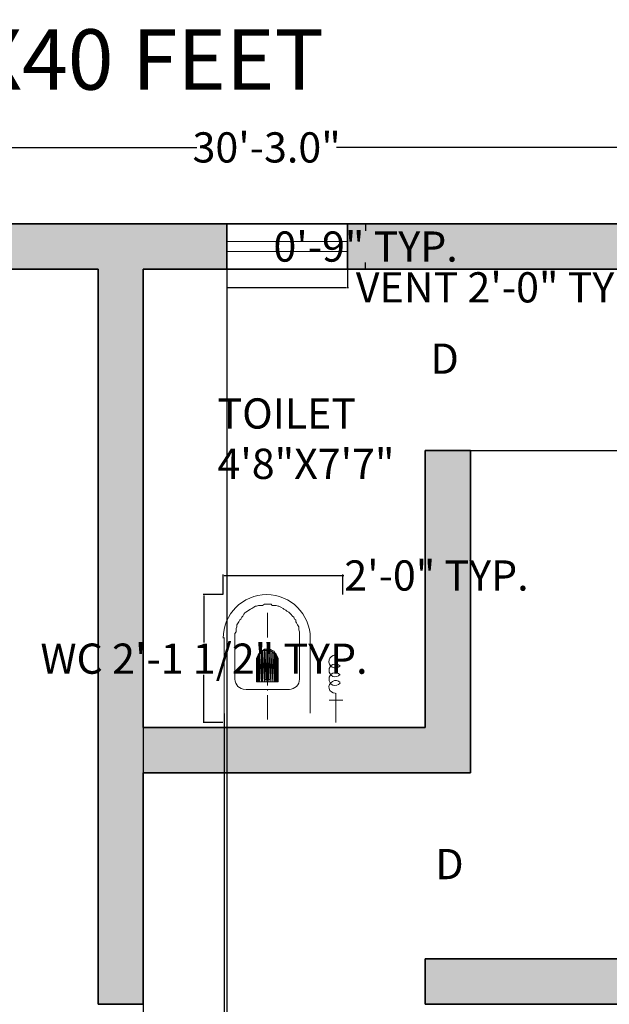
# Model space of a CAD drawing. Units: inches. Extents: x 2552 to 3196, y 4736 to 5443.
# Tile 6 of 8: x 2824 to 2941, y 5136 to 5332. Entities that reach past the tile are written whole.
import ezdxf

# ---------------------------------------------------------------- set-up
doc = ezdxf.new("R2010")
doc.units = ezdxf.units.IN
doc.header["$MEASUREMENT"] = 0
for name, color, linetype, lineweight in [('A-ANNO-DIMS', 2, 'Continuous', 18), ('A-ANNO-TTLB', 7, 'Continuous', 25), ('A-AREA-IDEN', 7, 'Continuous', 18), ('A-DOOR-IDEN', 7, 'Continuous', 18), ('A-FLOR-FIXT', 7, 'Continuous', 18), ('A-GLAZ', 4, 'Continuous', 18), ('A-WALL', 7, 'Continuous', 35)]:
    doc.layers.add(name, color=color, linetype=linetype, lineweight=lineweight)
doc.layers.add('A-WALL-PATT', color=30, linetype='Continuous', lineweight=13, true_color=0xf8991e)
doc.styles.get("Standard").update_dxf_attribs({"font": 'arial.ttf'})
doc.dimstyles.get("Standard").update_dxf_attribs({"dimtxt": 6, "dimasz": 0.18, "dimexe": 0.18, "dimexo": 0.0625, "dimgap": 0.09, "dimtad": 0, "dimtih": 1, "dimtoh": 1, "dimdec": 1, "dimzin": 0, "dimdsep": 46, "dimlunit": 3, "dimtxsty": 'Standard', "dimcen": 0.09, "dimadec": 0, "dimazin": 0, "dimtfac": 1, "dimtdec": 1, "dimtofl": 0, "dimtmove": 0, "dimatfit": 3, "dimfxl": 1, "dimtolj": 1, "dimtzin": 0, "dimarcsym": 0})

# ---------------------------------------------------------------- blocks, each defined once
blk = doc.blocks.new('*D2')
at = {"layer": 'A-ANNO-DIMS', "color": 0, "lineweight": -2, "transparency": 16777216}
for p, q in [((2691.66, 5291.38), (2691.66, 5306.69)), ((2691.84, 5306.51), (2859.27, 5306.51)), ((3054.48, 5306.51), (2887.04, 5306.51)), ((3054.66, 5291.38), (3054.66, 5306.69))]:
    blk.add_line(p, q, dxfattribs=at)
at = {"layer": 'A-ANNO-DIMS', "color": 0, "transparency": 16777216}
for points in [[(2691.84, 5306.54), (2691.84, 5306.48), (2691.66, 5306.51)], [(3054.48, 5306.54), (3054.48, 5306.48), (3054.66, 5306.51)]]:
    blk.add_solid(points, dxfattribs=at)
at = {"layer": 'Defpoints', "color": 0, "transparency": 16777216}
for p in [(3054.66, 5306.51), (2691.66, 5291.32), (3054.66, 5291.32)]:
    blk.add_point(p, dxfattribs=at)
at = {"layer": 'A-ANNO-DIMS', "color": 0, "transparency": 16777216, "insert": (2873.16, 5306.51), "char_height": 6, "attachment_point": 5}
blk.add_mtext('\\A1;30\'-3.0"', dxfattribs=at)
blk = doc.blocks.new('VENT-24IN')
for p, q in [((24, 9), (0, 9)), ((24, 5.5), (0, 5.5)), ((0, 3.5), (24, 3.5)), ((0, 0), (24, 0))]:
    blk.add_line(p, q)
blk = doc.blocks.new('WC-SQUAT')
h = blk.add_hatch(color=256)
h.paths.add_polyline_path([(7.21, 8.12), (7.21, 13.81), (7.05, 8.12)])
h.paths.add_polyline_path([(7.21, 13.81), (7.05, 8.12), (7.05, 13.58)])
h = blk.add_hatch(color=256)
h.paths.add_polyline_path([(7.59, 8.12), (7.59, 14.19), (7.21, 8.12)])
h.paths.add_polyline_path([(7.59, 14.19), (7.21, 8.12), (7.21, 13.81)])
h = blk.add_hatch(color=256)
h.paths.add_polyline_path([(7.81, 8.12), (7.81, 14.34), (7.59, 8.12)])
h.paths.add_polyline_path([(7.81, 14.34), (7.59, 8.12), (7.59, 14.19)])
h = blk.add_hatch(color=256)
h.paths.add_polyline_path([(8.19, 8.12), (8.19, 14.56), (7.81, 8.12)])
h.paths.add_polyline_path([(8.19, 14.56), (7.81, 8.12), (7.81, 14.34)])
h = blk.add_hatch(color=256)
h.paths.add_polyline_path([(8.57, 8.12), (8.57, 14.56), (8.19, 8.12)])
h.paths.add_polyline_path([(8.57, 14.56), (8.19, 8.12), (8.19, 14.56)])
h = blk.add_hatch(color=256)
h.paths.add_polyline_path([(8.95, 8.12), (8.95, 14.56), (8.57, 8.12)])
h.paths.add_polyline_path([(8.95, 14.56), (8.57, 8.12), (8.57, 14.56)])
h = blk.add_hatch(color=256)
h.paths.add_polyline_path([(9.33, 8.12), (9.33, 14.56), (8.95, 8.12)])
h.paths.add_polyline_path([(9.33, 14.56), (8.95, 8.12), (8.95, 14.56)])
h = blk.add_hatch(color=256)
h.paths.add_polyline_path([(9.71, 8.12), (9.71, 14.34), (9.33, 8.12)])
h.paths.add_polyline_path([(9.71, 14.34), (9.33, 8.12), (9.33, 14.56)])
h = blk.add_hatch(color=256)
h.paths.add_polyline_path([(10.16, 8.12), (10.16, 14.19), (9.71, 8.12)])
h.paths.add_polyline_path([(10.16, 14.19), (9.71, 8.12), (9.71, 14.34)])
h = blk.add_hatch(color=256)
h.paths.add_polyline_path([(10.32, 8.12), (10.32, 13.81), (10.16, 8.12)])
h.paths.add_polyline_path([(10.32, 13.81), (10.16, 8.12), (10.16, 14.19)])
h = blk.add_hatch(color=256)
h.paths.add_polyline_path([(10.54, 8.12), (10.54, 13.58), (10.32, 8.12)])
h.paths.add_polyline_path([(10.54, 13.58), (10.32, 8.12), (10.32, 13.81)])
h = blk.add_hatch(color=256)
h.paths.add_polyline_path([(6.83, 8.12), (6.83, 13.2), (6.6, 8.12)])
h.paths.add_polyline_path([(6.83, 13.2), (6.6, 8.12), (6.6, 12.82)])
h.paths.add_polyline_path([(6.6, 8.12), (6.6, 12.82), (6.6, 12.44)])
h = blk.add_hatch(color=256)
h.paths.add_polyline_path([(7.05, 8.12), (7.05, 13.58), (6.83, 8.12)])
h.paths.add_polyline_path([(7.05, 13.58), (6.83, 8.12), (6.83, 13.2)])
h = blk.add_hatch(color=256)
h.paths.add_polyline_path([(10.7, 8.12), (10.7, 13.2), (10.54, 8.12)])
h.paths.add_polyline_path([(10.7, 13.2), (10.54, 8.12), (10.54, 13.58)])
h = blk.add_hatch(color=256)
h.paths.add_polyline_path([(10.92, 8.12), (10.92, 12.82), (10.7, 8.12)])
h.paths.add_polyline_path([(10.92, 12.82), (10.7, 8.12), (10.7, 13.2)])
for points in [[(2.35, 15.93), (2.35, 16.69), (2.35, 17.3), (2.35, 17.67), (2.58, 18.05), (2.58, 18.43), (2.58, 18.66), (2.73, 19.04), (2.73, 19.42), (2.96, 19.8), (3.11, 20.03), (3.34, 20.41), (3.49, 20.56), (3.72, 20.94), (3.94, 21.16), (4.1, 21.54), (4.32, 21.77), (4.48, 21.92), (4.85, 22.15), (5.08, 22.3), (5.46, 22.53), (5.69, 22.68), (6.07, 22.91), (6.45, 23.14), (6.6, 23.14), (7.05, 23.29), (7.43, 23.29), (7.81, 23.29), (8.19, 23.52), (8.8, 23.52), (9.56, 23.52), (9.71, 23.29), (10.16, 23.29), (10.54, 23.29), (10.92, 23.14), (11.08, 23.14), (11.45, 22.91), (11.91, 22.68), (12.06, 22.53), (12.44, 22.3), (12.67, 22.15), (13.05, 21.92), (13.2, 21.77), (13.43, 21.54), (13.81, 21.16), (14.03, 20.94), (14.19, 20.56), (14.41, 20.41), (14.41, 20.03), (14.56, 19.8), (14.79, 19.42), (15.02, 19.04), (15.02, 18.66), (15.02, 18.43), (15.17, 18.05), (15.17, 17.67), (15.17, 17.3), (15.17, 16.69), (15.17, 15.93)], [(8.8, 16.92), (8.8, 21.77), (8.8, 21.77)], [(0.23, 1.9), (0.23, 16.92), (0.23, 16.92)], [(2.35, 8.72), (2.35, 15.93), (2.35, 15.93)], [(15.17, 8.72), (15.17, 15.93), (15.17, 15.93)], [(17.3, 1.9), (17.3, 16.92), (17.3, 16.92)], [(8.8, 7.36), (8.8, 14.94), (8.8, 14.94)], [(6.6, 8.12), (6.6, 12.44), (6.6, 12.44)], [(10.92, 8.12), (10.92, 12.44), (10.92, 12.44)], [(6.6, 8.12), (10.92, 8.12), (10.92, 8.12)], [(8.34, 8.57), (8.57, 8.57), (8.8, 8.57)], [(8.34, 8.57), (8.34, 8.5), (8.34, 8.5)], [(8.8, 8.57), (8.72, 8.5), (8.72, 8.5)], [(8.8, 8.57), (8.95, 8.57), (9.18, 8.57)], [(9.18, 8.57), (9.18, 8.5), (9.18, 8.5)], [(4.48, 6.6), (13.2, 6.6), (13.2, 6.6)], [(8.8, 6.37), (8.72, 6.37), (8.72, 6.37)], [(8.8, 0.61), (8.8, 5.46), (8.8, 5.46)], [(21.04, 4.48), (23.77, 4.48), (23.77, 4.48)], [(22.4, 0), (22.4, 5.84), (22.4, 5.84)]]:
    blk.add_lwpolyline(points)
for points in [[(7.21, 8.12), (7.21, 13.81), (7.05, 8.12)], [(7.21, 13.81), (7.05, 8.12), (7.05, 13.58)], [(7.59, 8.12), (7.59, 14.19), (7.21, 8.12)], [(7.59, 14.19), (7.21, 8.12), (7.21, 13.81)], [(7.81, 8.12), (7.81, 14.34), (7.59, 8.12)], [(7.81, 14.34), (7.59, 8.12), (7.59, 14.19)], [(8.19, 8.12), (8.19, 14.56), (7.81, 8.12)], [(8.19, 14.56), (7.81, 8.12), (7.81, 14.34)], [(8.57, 8.12), (8.57, 14.56), (8.19, 8.12)], [(8.57, 14.56), (8.19, 8.12), (8.19, 14.56)], [(8.95, 8.12), (8.95, 14.56), (8.57, 8.12)], [(8.95, 14.56), (8.57, 8.12), (8.57, 14.56)], [(9.33, 8.12), (9.33, 14.56), (8.95, 8.12)], [(9.33, 14.56), (8.95, 8.12), (8.95, 14.56)], [(9.71, 14.34), (9.33, 8.12), (9.33, 14.56)], [(9.71, 8.12), (9.71, 14.34), (9.33, 8.12)], [(10.16, 14.19), (9.71, 8.12), (9.71, 14.34)], [(10.16, 8.12), (10.16, 14.19), (9.71, 8.12)], [(10.32, 13.81), (10.16, 8.12), (10.16, 14.19)], [(10.32, 8.12), (10.32, 13.81), (10.16, 8.12)], [(10.54, 13.58), (10.32, 8.12), (10.32, 13.81)], [(6.83, 8.12), (6.83, 13.2), (6.6, 8.12)], [(6.83, 13.2), (6.6, 8.12), (6.6, 12.82)], [(6.6, 8.12), (6.6, 12.82), (6.6, 12.44)], [(6.6, 12.82), (6.6, 8.12), (6.6, 8.12)], [(7.05, 8.12), (7.05, 13.58), (6.83, 8.12)], [(7.05, 13.58), (6.83, 8.12), (6.83, 13.2)], [(10.54, 8.12), (10.54, 13.58), (10.32, 8.12)], [(10.7, 13.2), (10.54, 8.12), (10.54, 13.58)], [(10.7, 8.12), (10.7, 13.2), (10.54, 8.12)], [(10.92, 12.82), (10.7, 8.12), (10.7, 13.2)], [(10.92, 8.12), (10.92, 12.82), (10.7, 8.12)], [(10.92, 12.44), (10.92, 8.12), (10.92, 12.82)], [(10.92, 8.12), (10.92, 12.44)]]:
    blk.add_lwpolyline(points, close=True)
for points, knots in [([(17.3, 16.76), (17.3, 21.54), (13.43, 25.41), (8.65, 25.41), (8.65, 25.41), (3.87, 25.41), (0, 21.54), (0, 16.76)], [0, 0, 0, 0, 0.125, 0.125, 0.125, 0.125001, 1, 1, 1, 1]), ([(10.7, 12.29), (10.7, 13.43), (9.79, 14.34), (8.65, 14.34), (8.65, 14.34), (7.51, 14.34), (6.6, 13.43), (6.6, 12.29)], [0, 0, 0, 0, 0.125, 0.125, 0.125, 0.125001, 1, 1, 1, 1]), ([(22.25, 13.43), (21.72, 13.43), (21.19, 12.97), (21.04, 12.44), (21.04, 12.44), (20.88, 11.91), (21.19, 11.3), (21.64, 11), (21.64, 11), (22.17, 10.77), (22.78, 10.85), (23.16, 11.23)], [0, 0, 0, 0, 0.083333, 0.083333, 0.083333, 0.083334, 0.166667, 0.166667, 0.166667, 0.166668, 1, 1, 1, 1]), ([(23.23, 11.23), (22.86, 11.61), (22.32, 11.76), (21.79, 11.53), (21.79, 11.53), (21.34, 11.38), (21.04, 10.92), (21.04, 10.39), (21.04, 10.39), (21.04, 9.86), (21.34, 9.41), (21.79, 9.18), (21.79, 9.18), (22.32, 9.03), (22.86, 9.18), (23.23, 9.56)], [0, 0, 0, 0, 0.0625, 0.0625, 0.0625, 0.062501, 0.125, 0.125, 0.125, 0.125001, 0.1875, 0.1875, 0.1875, 0.187501, 1, 1, 1, 1]), ([(23.16, 9.48), (22.86, 9.86), (22.25, 10.01), (21.79, 9.79), (21.79, 9.79), (21.34, 9.63), (21.04, 9.1), (21.04, 8.65), (21.04, 8.65), (21.04, 8.12), (21.34, 7.66), (21.79, 7.43), (21.79, 7.43), (22.32, 7.28), (22.86, 7.43), (23.23, 7.81)], [0, 0, 0, 0, 0.0625, 0.0625, 0.0625, 0.062501, 0.125, 0.125, 0.125, 0.125001, 0.1875, 0.1875, 0.1875, 0.187501, 1, 1, 1, 1]), ([(23.23, 7.96), (22.86, 8.34), (22.17, 8.5), (21.72, 8.19), (21.72, 8.19), (21.19, 7.89), (20.88, 7.36), (21.04, 6.75), (21.04, 6.75), (21.19, 6.22), (21.72, 5.84), (22.25, 5.84)], [0, 0, 0, 0, 0.083333, 0.083333, 0.083333, 0.083334, 0.166667, 0.166667, 0.166667, 0.166668, 1, 1, 1, 1])]:
    blk.add_open_spline(points, degree=3, knots=knots)
for points in [[(2.35, 8.65), (2.35, 7.51), (3.26, 6.6), (4.4, 6.6)], [(13.12, 6.6), (14.26, 6.6), (15.17, 7.51), (15.17, 8.65)]]:
    blk.add_open_spline(points, degree=3)
blk = doc.blocks.new('*D11')
at = {"layer": 'A-ANNO-DIMS', "color": 0, "lineweight": -2, "transparency": 16777216}
for p, q in [((2865.22, 5282.26), (2865.22, 5278.54)), ((2889.22, 5282.26), (2889.22, 5278.54)), ((2865.4, 5278.72), (2889.04, 5278.72)), ((2889.22, 5278.72), (2889.4, 5278.72))]:
    blk.add_line(p, q, dxfattribs=at)
at = {"layer": 'A-ANNO-DIMS', "color": 0, "transparency": 16777216}
for points in [[(2865.4, 5278.75), (2865.4, 5278.69), (2865.22, 5278.72)], [(2889.04, 5278.75), (2889.04, 5278.69), (2889.22, 5278.72)]]:
    blk.add_solid(points, dxfattribs=at)
at = {"layer": 'Defpoints', "color": 0, "transparency": 16777216}
for p in [(2865.22, 5282.32), (2889.22, 5282.32), (2889.22, 5278.72)]:
    blk.add_point(p, dxfattribs=at)
at = {"layer": 'A-ANNO-DIMS', "color": 0, "transparency": 16777216, "insert": (2920.28, 5278.72), "char_height": 6, "attachment_point": 5}
blk.add_mtext('\\A1;VENT 2\'-0" TYP.', dxfattribs=at)
blk = doc.blocks.new('*D12')
at = {"layer": 'A-ANNO-DIMS', "color": 0, "lineweight": -2, "transparency": 16777216}
for p, q in [((2889.29, 5291.32), (2893, 5291.32)), ((2892.82, 5291.14), (2892.82, 5289.97)), ((2889.29, 5282.32), (2893, 5282.32)), ((2892.82, 5282.5), (2892.82, 5283.66))]:
    blk.add_line(p, q, dxfattribs=at)
at = {"layer": 'A-ANNO-DIMS', "color": 0, "transparency": 16777216}
for points in [[(2892.79, 5291.14), (2892.85, 5291.14), (2892.82, 5291.32)], [(2892.79, 5282.5), (2892.85, 5282.5), (2892.82, 5282.32)]]:
    blk.add_solid(points, dxfattribs=at)
at = {"layer": 'Defpoints', "color": 0, "transparency": 16777216}
for p in [(2889.22, 5291.32), (2892.82, 5291.32), (2889.22, 5282.32)]:
    blk.add_point(p, dxfattribs=at)
at = {"layer": 'A-ANNO-DIMS', "color": 0, "transparency": 16777216, "insert": (2892.82, 5286.82), "char_height": 6, "attachment_point": 5}
blk.add_mtext('\\A1;0\'-9" TYP.', dxfattribs=at)
blk = doc.blocks.new('*D15')
at = {"layer": 'A-ANNO-DIMS', "color": 0, "lineweight": -2, "transparency": 16777216}
for p, q in [((2864.46, 5217.68), (2860.53, 5217.68)), ((2860.71, 5217.5), (2860.71, 5208.17)), ((2860.71, 5192.45), (2860.71, 5201.78)), ((2864.46, 5192.27), (2860.53, 5192.27))]:
    blk.add_line(p, q, dxfattribs=at)
at = {"layer": 'A-ANNO-DIMS', "color": 0, "transparency": 16777216}
for points in [[(2860.68, 5217.5), (2860.74, 5217.5), (2860.71, 5217.68)], [(2860.68, 5192.45), (2860.74, 5192.45), (2860.71, 5192.27)]]:
    blk.add_solid(points, dxfattribs=at)
at = {"layer": 'Defpoints', "color": 0, "transparency": 16777216}
for p in [(2860.71, 5217.68), (2864.52, 5217.68), (2864.52, 5192.27)]:
    blk.add_point(p, dxfattribs=at)
at = {"layer": 'A-ANNO-DIMS', "color": 0, "transparency": 16777216, "insert": (2860.71, 5204.97), "char_height": 6, "attachment_point": 5}
blk.add_mtext('\\A1;WC 2\'-1 1/2" TYP.', dxfattribs=at)
blk = doc.blocks.new('*D16')
at = {"layer": 'A-ANNO-DIMS', "color": 0, "lineweight": -2, "transparency": 16777216}
for p, q in [((2864.52, 5217.74), (2864.52, 5221.67)), ((2864.7, 5221.49), (2888.11, 5221.49)), ((2888.29, 5217.74), (2888.29, 5221.67)), ((2888.29, 5221.49), (2888.47, 5221.49))]:
    blk.add_line(p, q, dxfattribs=at)
at = {"layer": 'A-ANNO-DIMS', "color": 0, "transparency": 16777216}
for points in [[(2864.7, 5221.52), (2864.7, 5221.46), (2864.52, 5221.49)], [(2888.11, 5221.52), (2888.11, 5221.46), (2888.29, 5221.49)]]:
    blk.add_solid(points, dxfattribs=at)
at = {"layer": 'Defpoints', "color": 0, "transparency": 16777216}
for p in [(2888.29, 5221.49), (2864.52, 5217.68), (2888.29, 5217.68)]:
    blk.add_point(p, dxfattribs=at)
at = {"layer": 'A-ANNO-DIMS', "color": 0, "transparency": 16777216, "insert": (2906.9, 5221.49), "char_height": 6, "attachment_point": 5}
blk.add_mtext('\\A1;2\'-0" TYP.', dxfattribs=at)
blk = doc.blocks.new('*D31')
at = {"layer": 'A-ANNO-DIMS', "color": 0, "lineweight": -2, "transparency": 16777216}
for p, q in [((2848.66, 5282.26), (2848.66, 4759.59)), ((2865.22, 5282.26), (2865.22, 4759.59)), ((2848.84, 4759.77), (2865.04, 4759.77)), ((2865.22, 4759.77), (2865.4, 4759.77))]:
    blk.add_line(p, q, dxfattribs=at)
at = {"layer": 'A-ANNO-DIMS', "color": 0, "transparency": 16777216}
for points in [[(2848.84, 4759.8), (2848.84, 4759.74), (2848.66, 4759.77)], [(2865.04, 4759.8), (2865.04, 4759.74), (2865.22, 4759.77)]]:
    blk.add_solid(points, dxfattribs=at)
at = {"layer": 'Defpoints', "color": 0, "transparency": 16777216}
for p in [(2848.66, 5282.32), (2865.22, 5282.32), (2865.22, 4759.77)]:
    blk.add_point(p, dxfattribs=at)
at = {"layer": 'A-ANNO-DIMS', "color": 0, "transparency": 16777216, "insert": (2880.18, 4759.77), "char_height": 6, "attachment_point": 5}
blk.add_mtext('\\A1;1\'-4 1/2"', dxfattribs=at)
blk = doc.blocks.new('*D32')
at = {"layer": 'A-ANNO-DIMS', "color": 0, "lineweight": -2, "transparency": 16777216}
for p, q in [((2864.75, 5194.1), (2864.75, 4759.59)), ((2848.66, 5191.26), (2848.66, 4759.59)), ((2848.48, 4759.77), (2848.3, 4759.77)), ((2864.93, 4759.77), (2865.11, 4759.77))]:
    blk.add_line(p, q, dxfattribs=at)
at = {"layer": 'A-ANNO-DIMS', "color": 0, "transparency": 16777216}
for points in [[(2848.48, 4759.8), (2848.48, 4759.74), (2848.66, 4759.77)], [(2864.93, 4759.8), (2864.93, 4759.74), (2864.75, 4759.77)]]:
    blk.add_solid(points, dxfattribs=at)
at = {"layer": 'Defpoints', "color": 0, "transparency": 16777216}
for p in [(2864.75, 5194.17), (2848.66, 5191.32), (2864.75, 4759.77)]:
    blk.add_point(p, dxfattribs=at)
at = {"layer": 'A-ANNO-DIMS', "color": 0, "transparency": 16777216, "insert": (2856.7, 4759.77), "char_height": 6, "attachment_point": 5}
blk.add_mtext('\\A1;1\'-4"', dxfattribs=at)
blk = doc.blocks.new('*D44')
at = {"layer": 'A-ANNO-DIMS', "color": 0, "lineweight": -2, "transparency": 16777216}
for p, q in [((2889.29, 5282.32), (3083.39, 5282.32)), ((3083.21, 5282.14), (3083.21, 5267.47)), ((3083.21, 5246.5), (3083.21, 5261.16)), ((2904.72, 5246.32), (3083.39, 5246.32))]:
    blk.add_line(p, q, dxfattribs=at)
at = {"layer": 'A-ANNO-DIMS', "color": 0, "transparency": 16777216}
for points in [[(3083.18, 5282.14), (3083.24, 5282.14), (3083.21, 5282.32)], [(3083.18, 5246.5), (3083.24, 5246.5), (3083.21, 5246.32)]]:
    blk.add_solid(points, dxfattribs=at)
at = {"layer": 'Defpoints', "color": 0, "transparency": 16777216}
for p in [(2889.22, 5282.32), (2904.66, 5246.32), (3083.21, 5246.32)]:
    blk.add_point(p, dxfattribs=at)
at = {"layer": 'A-ANNO-DIMS', "color": 0, "transparency": 16777216, "insert": (3083.21, 5264.32), "char_height": 6, "attachment_point": 5}
blk.add_mtext('\\A1;3\'-0"', dxfattribs=at)

msp = doc.modelspace()

# ---------------------------------------------------------------- hatches: boundary and pattern name
at = {"layer": 'A-WALL-PATT'}
h = msp.add_hatch(color=256, dxfattribs=at)
h.dxf.hatch_style = 1
h.paths.add_polyline_path([(2700.66, 5282.32), (2732.91, 5282.32), (2732.91, 5291.32), (2691.66, 5291.32), (2691.66, 5248.4), (2700.66, 5248.4)])
h.paths.add_polyline_path([(2865.22, 5291.32), (2792.91, 5291.32), (2792.91, 5282.32), (2839.66, 5282.32), (2839.66, 5136.32), (2848.66, 5136.32), (2848.66, 5182.32), (2913.66, 5182.32), (2913.66, 5246.32), (2904.66, 5246.32), (2904.66, 5191.32), (2848.66, 5191.32), (2848.66, 5282.32), (2865.22, 5282.32)])
h.paths.add_polyline_path([(2946.08, 5291.32), (2889.22, 5291.32), (2889.22, 5282.32), (2946.08, 5282.32)])
h.paths.add_polyline_path([(3054.66, 5291.32), (3006.08, 5291.32), (3006.08, 5282.32), (3045.66, 5282.32), (3045.66, 5249.18), (3054.66, 5249.18)])
h.paths.add_polyline_path([(3054.66, 5189.18), (3045.66, 5189.18), (3045.66, 5145.32), (2904.66, 5145.32), (2904.66, 5136.32), (3045.66, 5136.32), (3045.66, 5103.54), (3054.66, 5103.54)])
h.paths.add_polyline_path([(3054.66, 5043.54), (3045.66, 5043.54), (3045.66, 5012.32), (2913.66, 5012.32), (2913.66, 5100.32), (2904.66, 5100.32), (2904.66, 5003.32), (3045.66, 5003.32), (3045.66, 4980.34), (3054.66, 4980.34)])
h.paths.add_polyline_path([(3054.66, 4920.34), (3045.66, 4920.34), (3045.66, 4886.32), (3029.6, 4886.32), (3029.6, 4877.32), (3045.66, 4877.32), (3045.66, 4817.32), (3041.59, 4817.32), (3041.59, 4808.32), (3054.66, 4808.32)])
h.paths.add_polyline_path([(2996.66, 4877.32), (3013.11, 4877.32), (3013.11, 4886.32), (2987.66, 4886.32), (2987.66, 4808.32), (2999.73, 4808.32), (2999.73, 4817.32), (2996.66, 4817.32)])
h.paths.add_polyline_path([(2825.66, 4877.32), (2853.9, 4877.32), (2853.9, 4886.32), (2825.66, 4886.32), (2825.66, 5000.12), (2816.66, 5000.12), (2816.66, 4817.32), (2785.76, 4817.32), (2785.76, 4808.32), (2825.66, 4808.32)])
h.paths.add_polyline_path([(2951.66, 4886.32), (2913.9, 4886.32), (2913.9, 4877.32), (2951.66, 4877.32)])
h.paths.add_polyline_path([(2725.76, 4817.32), (2700.66, 4817.32), (2700.66, 4833.17), (2691.66, 4833.17), (2691.66, 4808.32), (2725.76, 4808.32)])
h.paths.add_polyline_path([(2700.66, 4902.32), (2691.66, 4902.32), (2691.66, 4869.17), (2700.66, 4869.17)])
h.paths.add_polyline_path([(2765.91, 4947.32), (2700.66, 4947.32), (2700.66, 4977.71), (2691.66, 4977.71), (2691.66, 4938.32), (2765.91, 4938.32)])
h.paths.add_polyline_path([(2825.66, 5077.32), (2773.66, 5077.32), (2773.66, 5112.32), (2764.66, 5112.32), (2764.66, 5077.32), (2700.66, 5077.32), (2700.66, 5102.51), (2691.66, 5102.51), (2691.66, 5037.71), (2700.66, 5037.71), (2700.66, 5068.32), (2816.66, 5068.32), (2816.66, 5036.12), (2825.66, 5036.12)])
h.paths.add_polyline_path([(2803.66, 5145.32), (2700.66, 5145.32), (2700.66, 5188.4), (2691.66, 5188.4), (2691.66, 5126.51), (2700.66, 5126.51), (2700.66, 5136.32), (2803.66, 5136.32)])

# ---------------------------------------------------------------- linework, layer by layer
at = {"layer": 'A-WALL'}
for p, q in [((2691.66, 5291.32), (3054.66, 5291.32)), ((2865.22, 5291.32), (2865.22, 5282.32)), ((2889.22, 5282.32), (2889.22, 5291.32)), ((2700.66, 5282.32), (2839.66, 5282.32)), ((2839.66, 5282.32), (2839.66, 5136.32)), ((2848.66, 5282.32), (2848.66, 5191.32)), ((2848.66, 5282.32), (3045.66, 5282.32)), ((2913.66, 5282.32), (2913.66, 5282.32)), ((2913.66, 5246.32), (2904.66, 5246.32)), ((2904.66, 5246.32), (2904.66, 5191.32)), ((2913.66, 5246.32), (2913.66, 5182.32)), ((2848.66, 5191.32), (2904.66, 5191.32)), ((2848.66, 5182.32), (2913.66, 5182.32)), ((2848.66, 5182.32), (2848.66, 5136.32)), ((2904.66, 5145.32), (3045.66, 5145.32)), ((2904.66, 5145.32), (2904.66, 5136.32)), ((2839.66, 5136.32), (2848.66, 5136.32)), ((2904.66, 5136.32), (3045.66, 5136.32))]:
    msp.add_line(p, q, dxfattribs=at)

# ---------------------------------------------------------------- block references
at = {"layer": 'A-FLOR-FIXT'}
msp.add_blockref('WC-SQUAT', (2864.52, 5192.27), dxfattribs=at)
at = {"layer": 'A-GLAZ'}
msp.add_blockref('VENT-24IN', (2865.22, 5282.32), dxfattribs=at)

# ---------------------------------------------------------------- texts
at = {"layer": 'A-ANNO-TTLB', "insert": (2760.34, 5349.98), "char_height": 12, "attachment_point": 1}
msp.add_mtext_dynamic_manual_height_columns('EAST FACING HOUSE PLAN\\P          30X40 FEET', width=240.3543, gutter_width=1, heights=[0], dxfattribs=at)
at = {"layer": 'A-AREA-IDEN', "insert": (2863.39, 5256.67), "char_height": 6, "attachment_point": 1}
msp.add_mtext_dynamic_manual_height_columns('TOILET\\P4\'8"X7\'7"', width=51.2884, gutter_width=1, heights=[0], dxfattribs=at)
at = {"layer": 'A-DOOR-IDEN', "char_height": 6, "attachment_point": 1}
for insert in [(2905.72, 5267.55), (2906.67, 5167.17)]:
    msp.add_mtext_dynamic_manual_height_columns('D', width=10.2167, gutter_width=1, heights=[0], dxfattribs=dict(at, insert=insert))

# ---------------------------------------------------------------- dimensions: what is measured, and where the dimension line sits
at = {"layer": 'A-ANNO-DIMS'}
for base, p1, p2, override, picture, middle in [((3054.66, 5306.51), (2691.66, 5291.32), (3054.66, 5291.32), {"dimclrd": 0, "dimclre": 0, "dimclrt": 0}, '*D2', (2873.16, 5306.51)), ((2865.22, 4759.77), (2848.66, 5282.32), (2865.22, 5282.32), {"dimdec": 1, "dimlfac": 1, "dimrnd": 0, "dimzin": 1, "dimdsep": 46, "dimlunit": 4, "dimfrac": 2}, '*D31', (2880.18, 4759.77)), ((2864.75, 4759.77), (2848.66, 5191.32), (2864.75, 5194.17), {"dimdec": 1, "dimlfac": 1, "dimrnd": 0, "dimzin": 1, "dimdsep": 46, "dimlunit": 4, "dimfrac": 2}, '*D32', (2856.7, 4759.77))]:
    dim = msp.add_linear_dim(base=base, p1=p1, p2=p2, dimstyle='Standard', override=override, dxfattribs=at)
    dim.commit()
    dim.dimension.update_dxf_attribs({"geometry": picture, "text_midpoint": middle})
for base, p1, p2, text, picture, middle in [((2892.82, 5291.32), (2889.22, 5282.32), (2889.22, 5291.32), '<> TYP.', '*D12', (2892.82, 5286.82)), ((2860.71, 5217.68), (2864.52, 5192.27), (2864.52, 5217.68), 'WC <> TYP.', '*D15', (2860.71, 5204.97))]:
    dim = msp.add_linear_dim(base=base, p1=p1, p2=p2, angle=90, text=text, dimstyle='Standard', override={"dimdec": 1, "dimlfac": 1, "dimrnd": 0, "dimzin": 1, "dimdsep": 46, "dimlunit": 4, "dimfrac": 2}, dxfattribs=at)
    dim.commit()
    dim.dimension.update_dxf_attribs({"geometry": picture, "text_midpoint": middle})
for base, p1, p2, text, picture, middle in [((2889.22, 5278.72), (2865.22, 5282.32), (2889.22, 5282.32), 'VENT <> TYP.', '*D11', (2920.28, 5278.72)), ((2888.29, 5221.49), (2864.52, 5217.68), (2888.29, 5217.68), '<> TYP.', '*D16', (2906.9, 5221.49))]:
    dim = msp.add_linear_dim(base=base, p1=p1, p2=p2, text=text, dimstyle='Standard', override={"dimdec": 1, "dimlfac": 1, "dimrnd": 0, "dimzin": 1, "dimdsep": 46, "dimlunit": 4, "dimfrac": 2}, dxfattribs=at)
    dim.commit()
    dim.dimension.update_dxf_attribs({"geometry": picture, "text_midpoint": middle})
dim = msp.add_linear_dim(base=(3083.21, 5246.32), p1=(2889.22, 5282.32), p2=(2904.66, 5246.32), angle=90, dimstyle='Standard', override={"dimdec": 1, "dimlfac": 1, "dimrnd": 0, "dimzin": 1, "dimdsep": 46, "dimlunit": 4, "dimfrac": 2}, dxfattribs=at)
dim.commit()
dim.dimension.update_dxf_attribs({"geometry": '*D44', "text_midpoint": (3083.21, 5264.32)})

doc.saveas('drawing.dxf')
